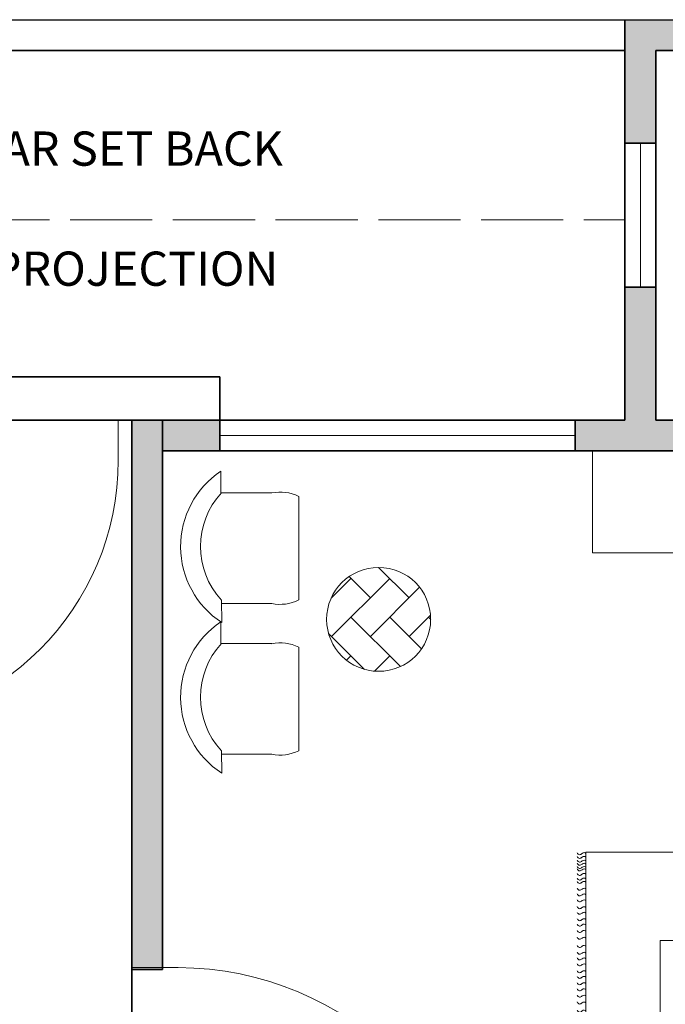
# Model space of a CAD drawing. Units: inches. Extents: x 0 to 4258, y 0 to 3769.
# Tile 27 of 30: x 3845 to 3940, y 3513 to 3657. Entities that reach past the tile are written whole.
import ezdxf

# ---------------------------------------------------------------- set-up
doc = ezdxf.new("R2010")
doc.units = ezdxf.units.IN
doc.header["$MEASUREMENT"] = 0
doc.linetypes.add('ACAD_ISO02W100', pattern=[15, 12, -3])
doc.layers.get('0').update_dxf_attribs({"color": 16})
for name, color, linetype, lineweight in [('A-ANNO-TEXT', 250, 'Continuous', 18), ('A-FLOR-OVHD', 150, 'ACAD_ISO02W100', 13), ('A-WALL-PATT', 16, 'Continuous', 13), ('C-PROP', 150, 'Continuous', 25), ('doors', 250, 'Continuous', 18), ('furniture', 13, 'Continuous', 18), ('walls', 251, 'Continuous', 35), ('windows', 121, 'Continuous', 18)]:
    doc.layers.add(name, color=color, linetype=linetype, lineweight=lineweight)
doc.styles.get("Standard").update_dxf_attribs({"font": 'arial.ttf'})

# ---------------------------------------------------------------- blocks, each defined once
blk = doc.blocks.new('CARPET')
at = {"layer": 'furniture'}
for p, q in [((-51.53, -98.11), (-51.53, -55.12)), ((-51.53, -55.12), (-41.27, -55.12)), ((36, -55.12), (51.55, -55.12)), ((51.55, -55.12), (51.55, -98.11)), ((51.55, -98.11), (-51.53, -98.11))]:
    blk.add_line(p, q, dxfattribs=at)
for points, knots in [([(-53.37, -55.99), (-53.22, -55.8), (-52.9, -55.41), (-52.34, -55.8), (-51.89, -56.08), (-51.65, -55.91), (-51.53, -55.83)], [0, 0, 0, 0, 0.653278, 1.290138, 1.740457, 2.114451, 2.114451, 2.114451, 2.114451]), ([(53.37, -55.99), (53.22, -55.8), (52.9, -55.41), (52.34, -55.8), (51.89, -56.08), (51.65, -55.91), (51.53, -55.83)], [0, 0, 0, 0, 0.653278, 1.290138, 1.740457, 2.114451, 2.114451, 2.114451, 2.114451]), ([(-53.37, -57.26), (-53.22, -57.07), (-52.9, -56.67), (-52.34, -57.07), (-51.89, -57.35), (-51.65, -57.17), (-51.53, -57.1)], [0, 0, 0, 0, 0.653278, 1.290138, 1.740457, 2.114451, 2.114451, 2.114451, 2.114451]), ([(53.37, -57.26), (53.22, -57.07), (52.9, -56.67), (52.34, -57.07), (51.89, -57.35), (51.65, -57.17), (51.53, -57.1)], [0, 0, 0, 0, 0.653278, 1.290138, 1.740457, 2.114451, 2.114451, 2.114451, 2.114451]), ([(-53.37, -58.59), (-53.22, -58.4), (-52.9, -58.01), (-52.34, -58.4), (-51.89, -58.68), (-51.65, -58.5), (-51.53, -58.43)], [0, 0, 0, 0, 0.653278, 1.290138, 1.740457, 2.114451, 2.114451, 2.114451, 2.114451]), ([(-53.37, -59.78), (-53.22, -59.58), (-52.9, -59.19), (-52.34, -59.58), (-51.89, -59.86), (-51.65, -59.69), (-51.53, -59.61)], [0, 0, 0, 0, 0.653278, 1.290138, 1.740457, 2.114451, 2.114451, 2.114451, 2.114451]), ([(53.37, -58.59), (53.22, -58.4), (52.9, -58.01), (52.34, -58.4), (51.89, -58.68), (51.65, -58.5), (51.53, -58.43)], [0, 0, 0, 0, 0.653278, 1.290138, 1.740457, 2.114451, 2.114451, 2.114451, 2.114451]), ([(53.37, -59.78), (53.22, -59.58), (52.9, -59.19), (52.34, -59.58), (51.89, -59.86), (51.65, -59.69), (51.53, -59.61)], [0, 0, 0, 0, 0.653278, 1.290138, 1.740457, 2.114451, 2.114451, 2.114451, 2.114451]), ([(-53.37, -61.22), (-53.22, -61.02), (-52.9, -60.63), (-52.34, -61.02), (-51.89, -61.3), (-51.65, -61.13), (-51.53, -61.05)], [0, 0, 0, 0, 0.653278, 1.290138, 1.740457, 2.114451, 2.114451, 2.114451, 2.114451]), ([(53.37, -61.22), (53.22, -61.02), (52.9, -60.63), (52.34, -61.02), (51.89, -61.3), (51.65, -61.13), (51.53, -61.05)], [0, 0, 0, 0, 0.653278, 1.290138, 1.740457, 2.114451, 2.114451, 2.114451, 2.114451]), ([(-53.37, -62.44), (-53.22, -62.25), (-52.9, -61.86), (-52.34, -62.25), (-51.89, -62.53), (-51.65, -62.36), (-51.53, -62.28)], [0, 0, 0, 0, 0.653278, 1.290138, 1.740457, 2.114451, 2.114451, 2.114451, 2.114451]), ([(-53.37, -63.63), (-53.22, -63.43), (-52.9, -63.04), (-52.34, -63.43), (-51.89, -63.72), (-51.65, -63.54), (-51.53, -63.46)], [0, 0, 0, 0, 0.653278, 1.290138, 1.740457, 2.114451, 2.114451, 2.114451, 2.114451]), ([(53.37, -62.44), (53.22, -62.25), (52.9, -61.86), (52.34, -62.25), (51.89, -62.53), (51.65, -62.36), (51.53, -62.28)], [0, 0, 0, 0, 0.653278, 1.290138, 1.740457, 2.114451, 2.114451, 2.114451, 2.114451]), ([(53.37, -63.63), (53.22, -63.43), (52.9, -63.04), (52.34, -63.43), (51.89, -63.72), (51.65, -63.54), (51.53, -63.46)], [0, 0, 0, 0, 0.653278, 1.290138, 1.740457, 2.114451, 2.114451, 2.114451, 2.114451]), ([(-53.37, -65.07), (-53.22, -64.87), (-52.9, -64.48), (-52.34, -64.87), (-51.89, -65.15), (-51.65, -64.98), (-51.53, -64.9)], [0, 0, 0, 0, 0.653278, 1.290138, 1.740457, 2.114451, 2.114451, 2.114451, 2.114451]), ([(53.37, -65.07), (53.22, -64.87), (52.9, -64.48), (52.34, -64.87), (51.89, -65.15), (51.65, -64.98), (51.53, -64.9)], [0, 0, 0, 0, 0.653278, 1.290138, 1.740457, 2.114451, 2.114451, 2.114451, 2.114451]), ([(-53.37, -66.76), (-53.22, -66.56), (-52.9, -66.17), (-52.34, -66.56), (-51.89, -66.84), (-51.65, -66.67), (-51.53, -66.59)], [0, 0, 0, 0, 0.653278, 1.290138, 1.740457, 2.114451, 2.114451, 2.114451, 2.114451]), ([(-53.37, -68.2), (-53.22, -68), (-52.9, -67.61), (-52.34, -68), (-51.89, -68.28), (-51.65, -68.11), (-51.53, -68.03)], [0, 0, 0, 0, 0.653278, 1.290138, 1.740457, 2.114451, 2.114451, 2.114451, 2.114451]), ([(53.37, -66.76), (53.22, -66.56), (52.9, -66.17), (52.34, -66.56), (51.89, -66.84), (51.65, -66.67), (51.53, -66.59)], [0, 0, 0, 0, 0.653278, 1.290138, 1.740457, 2.114451, 2.114451, 2.114451, 2.114451]), ([(53.37, -68.2), (53.22, -68), (52.9, -67.61), (52.34, -68), (51.89, -68.28), (51.65, -68.11), (51.53, -68.03)], [0, 0, 0, 0, 0.653278, 1.290138, 1.740457, 2.114451, 2.114451, 2.114451, 2.114451]), ([(-53.37, -69.53), (-53.22, -69.33), (-52.9, -68.94), (-52.34, -69.33), (-51.89, -69.61), (-51.65, -69.44), (-51.53, -69.36)], [0, 0, 0, 0, 0.653278, 1.290138, 1.740457, 2.114451, 2.114451, 2.114451, 2.114451]), ([(53.37, -69.53), (53.22, -69.33), (52.9, -68.94), (52.34, -69.33), (51.89, -69.61), (51.65, -69.44), (51.53, -69.36)], [0, 0, 0, 0, 0.653278, 1.290138, 1.740457, 2.114451, 2.114451, 2.114451, 2.114451]), ([(-53.37, -70.79), (-53.22, -70.6), (-52.9, -70.21), (-52.34, -70.6), (-51.89, -70.88), (-51.65, -70.7), (-51.53, -70.63)], [0, 0, 0, 0, 0.653278, 1.290138, 1.740457, 2.114451, 2.114451, 2.114451, 2.114451]), ([(-53.37, -72.12), (-53.22, -71.93), (-52.9, -71.54), (-52.34, -71.93), (-51.89, -72.21), (-51.65, -72.04), (-51.53, -71.96)], [0, 0, 0, 0, 0.653278, 1.290138, 1.740457, 2.114451, 2.114451, 2.114451, 2.114451]), ([(53.37, -70.79), (53.22, -70.6), (52.9, -70.21), (52.34, -70.6), (51.89, -70.88), (51.65, -70.7), (51.53, -70.63)], [0, 0, 0, 0, 0.653278, 1.290138, 1.740457, 2.114451, 2.114451, 2.114451, 2.114451]), ([(53.37, -72.12), (53.22, -71.93), (52.9, -71.54), (52.34, -71.93), (51.89, -72.21), (51.65, -72.04), (51.53, -71.96)], [0, 0, 0, 0, 0.653278, 1.290138, 1.740457, 2.114451, 2.114451, 2.114451, 2.114451]), ([(-53.37, -73.31), (-53.22, -73.11), (-52.9, -72.72), (-52.34, -73.11), (-51.89, -73.4), (-51.65, -73.22), (-51.53, -73.14)], [0, 0, 0, 0, 0.653278, 1.290138, 1.740457, 2.114451, 2.114451, 2.114451, 2.114451]), ([(53.37, -73.31), (53.22, -73.11), (52.9, -72.72), (52.34, -73.11), (51.89, -73.4), (51.65, -73.22), (51.53, -73.14)], [0, 0, 0, 0, 0.653278, 1.290138, 1.740457, 2.114451, 2.114451, 2.114451, 2.114451]), ([(-53.37, -74.75), (-53.22, -74.55), (-52.9, -74.16), (-52.34, -74.55), (-51.89, -74.83), (-51.65, -74.66), (-51.53, -74.58)], [0, 0, 0, 0, 0.653278, 1.290138, 1.740457, 2.114451, 2.114451, 2.114451, 2.114451]), ([(-53.37, -75.98), (-53.22, -75.78), (-52.9, -75.39), (-52.34, -75.78), (-51.89, -76.06), (-51.65, -75.89), (-51.53, -75.81)], [0, 0, 0, 0, 0.653278, 1.290138, 1.740457, 2.114451, 2.114451, 2.114451, 2.114451]), ([(53.37, -74.75), (53.22, -74.55), (52.9, -74.16), (52.34, -74.55), (51.89, -74.83), (51.65, -74.66), (51.53, -74.58)], [0, 0, 0, 0, 0.653278, 1.290138, 1.740457, 2.114451, 2.114451, 2.114451, 2.114451]), ([(53.37, -75.98), (53.22, -75.78), (52.9, -75.39), (52.34, -75.78), (51.89, -76.06), (51.65, -75.89), (51.53, -75.81)], [0, 0, 0, 0, 0.653278, 1.290138, 1.740457, 2.114451, 2.114451, 2.114451, 2.114451]), ([(-53.37, -77.16), (-53.22, -76.96), (-52.9, -76.57), (-52.34, -76.96), (-51.89, -77.25), (-51.65, -77.07), (-51.53, -76.99)], [0, 0, 0, 0, 0.653278, 1.290138, 1.740457, 2.114451, 2.114451, 2.114451, 2.114451]), ([(-53.37, -78.6), (-53.22, -78.4), (-52.9, -78.01), (-52.34, -78.4), (-51.89, -78.68), (-51.65, -78.51), (-51.53, -78.43)], [0, 0, 0, 0, 0.653278, 1.290138, 1.740457, 2.114451, 2.114451, 2.114451, 2.114451]), ([(53.37, -77.16), (53.22, -76.96), (52.9, -76.57), (52.34, -76.96), (51.89, -77.25), (51.65, -77.07), (51.53, -76.99)], [0, 0, 0, 0, 0.653278, 1.290138, 1.740457, 2.114451, 2.114451, 2.114451, 2.114451]), ([(53.37, -78.6), (53.22, -78.4), (52.9, -78.01), (52.34, -78.4), (51.89, -78.68), (51.65, -78.51), (51.53, -78.43)], [0, 0, 0, 0, 0.653278, 1.290138, 1.740457, 2.114451, 2.114451, 2.114451, 2.114451]), ([(-53.37, -80.29), (-53.22, -80.09), (-52.9, -79.7), (-52.34, -80.09), (-51.89, -80.37), (-51.65, -80.2), (-51.53, -80.12)], [0, 0, 0, 0, 0.653278, 1.290138, 1.740457, 2.114451, 2.114451, 2.114451, 2.114451]), ([(53.37, -80.29), (53.22, -80.09), (52.9, -79.7), (52.34, -80.09), (51.89, -80.37), (51.65, -80.2), (51.53, -80.12)], [0, 0, 0, 0, 0.653278, 1.290138, 1.740457, 2.114451, 2.114451, 2.114451, 2.114451]), ([(-53.37, -81.73), (-53.22, -81.53), (-52.9, -81.14), (-52.34, -81.53), (-51.89, -81.81), (-51.65, -81.64), (-51.53, -81.56)], [0, 0, 0, 0, 0.653278, 1.290138, 1.740457, 2.114451, 2.114451, 2.114451, 2.114451]), ([(53.37, -81.73), (53.22, -81.53), (52.9, -81.14), (52.34, -81.53), (51.89, -81.81), (51.65, -81.64), (51.53, -81.56)], [0, 0, 0, 0, 0.653278, 1.290138, 1.740457, 2.114451, 2.114451, 2.114451, 2.114451]), ([(-53.37, -83.06), (-53.22, -82.86), (-52.9, -82.47), (-52.34, -82.86), (-51.89, -83.14), (-51.65, -82.97), (-51.53, -82.89)], [0, 0, 0, 0, 0.653278, 1.290138, 1.740457, 2.114451, 2.114451, 2.114451, 2.114451]), ([(-53.37, -84.18), (-53.22, -83.99), (-52.9, -83.6), (-52.34, -83.99), (-51.89, -84.27), (-51.65, -84.09), (-51.53, -84.02)], [0, 0, 0, 0, 0.653278, 1.290138, 1.740457, 2.114451, 2.114451, 2.114451, 2.114451]), ([(53.37, -83.06), (53.22, -82.86), (52.9, -82.47), (52.34, -82.86), (51.89, -83.14), (51.65, -82.97), (51.53, -82.89)], [0, 0, 0, 0, 0.653278, 1.290138, 1.740457, 2.114451, 2.114451, 2.114451, 2.114451]), ([(53.37, -84.18), (53.22, -83.99), (52.9, -83.6), (52.34, -83.99), (51.89, -84.27), (51.65, -84.09), (51.53, -84.02)], [0, 0, 0, 0, 0.653278, 1.290138, 1.740457, 2.114451, 2.114451, 2.114451, 2.114451]), ([(-53.37, -85.51), (-53.22, -85.32), (-52.9, -84.93), (-52.34, -85.32), (-51.89, -85.6), (-51.65, -85.42), (-51.53, -85.35)], [0, 0, 0, 0, 0.653278, 1.290138, 1.740457, 2.114451, 2.114451, 2.114451, 2.114451]), ([(-53.37, -86.7), (-53.22, -86.5), (-52.9, -86.11), (-52.34, -86.5), (-51.89, -86.78), (-51.65, -86.61), (-51.53, -86.53)], [0, 0, 0, 0, 0.653278, 1.290138, 1.740457, 2.114451, 2.114451, 2.114451, 2.114451]), ([(53.37, -85.51), (53.22, -85.32), (52.9, -84.93), (52.34, -85.32), (51.89, -85.6), (51.65, -85.42), (51.53, -85.35)], [0, 0, 0, 0, 0.653278, 1.290138, 1.740457, 2.114451, 2.114451, 2.114451, 2.114451]), ([(53.37, -86.7), (53.22, -86.5), (52.9, -86.11), (52.34, -86.5), (51.89, -86.78), (51.65, -86.61), (51.53, -86.53)], [0, 0, 0, 0, 0.653278, 1.290138, 1.740457, 2.114451, 2.114451, 2.114451, 2.114451]), ([(-53.37, -88.14), (-53.22, -87.94), (-52.9, -87.55), (-52.34, -87.94), (-51.89, -88.22), (-51.65, -88.05), (-51.53, -87.97)], [0, 0, 0, 0, 0.653278, 1.290138, 1.740457, 2.114451, 2.114451, 2.114451, 2.114451]), ([(53.37, -88.14), (53.22, -87.94), (52.9, -87.55), (52.34, -87.94), (51.89, -88.22), (51.65, -88.05), (51.53, -87.97)], [0, 0, 0, 0, 0.653278, 1.290138, 1.740457, 2.114451, 2.114451, 2.114451, 2.114451]), ([(-53.37, -89.36), (-53.22, -89.17), (-52.9, -88.78), (-52.34, -89.17), (-51.89, -89.45), (-51.65, -89.28), (-51.53, -89.2)], [0, 0, 0, 0, 0.653278, 1.290138, 1.740457, 2.114451, 2.114451, 2.114451, 2.114451]), ([(-53.37, -90.55), (-53.22, -90.35), (-52.9, -89.96), (-52.34, -90.35), (-51.89, -90.64), (-51.65, -90.46), (-51.53, -90.38)], [0, 0, 0, 0, 0.653278, 1.290138, 1.740457, 2.114451, 2.114451, 2.114451, 2.114451]), ([(53.37, -89.36), (53.22, -89.17), (52.9, -88.78), (52.34, -89.17), (51.89, -89.45), (51.65, -89.28), (51.53, -89.2)], [0, 0, 0, 0, 0.653278, 1.290138, 1.740457, 2.114451, 2.114451, 2.114451, 2.114451]), ([(53.37, -90.55), (53.22, -90.35), (52.9, -89.96), (52.34, -90.35), (51.9, -90.63), (51.66, -90.47), (51.55, -90.4)], [0, 0, 0, 0, 0.653278, 1.290138, 1.740457, 2.0926, 2.0926, 2.0926, 2.0926]), ([(-53.37, -91.99), (-53.22, -91.79), (-52.9, -91.4), (-52.34, -91.79), (-51.89, -92.07), (-51.65, -91.9), (-51.53, -91.82)], [0, 0, 0, 0, 0.653278, 1.290138, 1.740457, 2.114451, 2.114451, 2.114451, 2.114451]), ([(-53.37, -92.69), (-53.22, -92.48), (-52.9, -92.08), (-52.35, -92.49), (-51.89, -92.77), (-51.65, -92.6), (-51.53, -92.52)], [0, 0, 0, 0, 0.663904, 1.307406, 1.757725, 2.131719, 2.131719, 2.131719, 2.131719]), ([(53.37, -91.99), (53.22, -91.79), (52.9, -91.4), (52.34, -91.79), (51.9, -92.07), (51.66, -91.91), (51.55, -91.83)], [0, 0, 0, 0, 0.653278, 1.290138, 1.740457, 2.0926, 2.0926, 2.0926, 2.0926]), ([(53.37, -92.69), (53.22, -92.49), (52.9, -92.09), (52.34, -92.49), (51.9, -92.77), (51.66, -92.61), (51.55, -92.53)], [0, 0, 0, 0, 0.656792, 1.295826, 1.746145, 2.098292, 2.098292, 2.098292, 2.098292]), ([(-53.37, -93.61), (-53.22, -93.42), (-52.9, -93.03), (-52.34, -93.42), (-51.89, -93.7), (-51.65, -93.52), (-51.53, -93.45)], [0, 0, 0, 0, 0.653278, 1.290138, 1.740457, 2.114451, 2.114451, 2.114451, 2.114451]), ([(-53.37, -94.55), (-53.22, -94.35), (-52.9, -93.96), (-52.34, -94.35), (-51.89, -94.63), (-51.65, -94.46), (-51.53, -94.38)], [0, 0, 0, 0, 0.653278, 1.290138, 1.740457, 2.114451, 2.114451, 2.114451, 2.114451]), ([(-53.37, -95.05), (-53.22, -94.85), (-52.9, -94.46), (-52.34, -94.85), (-51.89, -95.14), (-51.65, -94.96), (-51.53, -94.88)], [0, 0, 0, 0, 0.653278, 1.290138, 1.740457, 2.114451, 2.114451, 2.114451, 2.114451]), ([(53.37, -93.66), (53.22, -93.46), (52.9, -93.07), (52.34, -93.46), (51.9, -93.74), (51.66, -93.58), (51.55, -93.5)], [0, 0, 0, 0, 0.653278, 1.290138, 1.740457, 2.0926, 2.0926, 2.0926, 2.0926]), ([(53.37, -94.59), (53.22, -94.4), (52.9, -94.01), (52.34, -94.4), (51.9, -94.68), (51.66, -94.51), (51.55, -94.44)], [0, 0, 0, 0, 0.653278, 1.290138, 1.740457, 2.0926, 2.0926, 2.0926, 2.0926]), ([(53.37, -95.1), (53.22, -94.9), (52.9, -94.51), (52.34, -94.9), (51.9, -95.18), (51.66, -95.02), (51.55, -94.94)], [0, 0, 0, 0, 0.653278, 1.290138, 1.740457, 2.0926, 2.0926, 2.0926, 2.0926]), ([(-53.37, -95.73), (-53.22, -95.54), (-52.9, -95.15), (-52.34, -95.54), (-51.89, -95.82), (-51.65, -95.65), (-51.53, -95.57)], [0, 0, 0, 0, 0.653278, 1.290138, 1.740457, 2.114451, 2.114451, 2.114451, 2.114451]), ([(-53.37, -96.38), (-53.22, -96.18), (-52.9, -95.79), (-52.34, -96.18), (-51.89, -96.47), (-51.65, -96.29), (-51.53, -96.21)], [0, 0, 0, 0, 0.653278, 1.290138, 1.740457, 2.114451, 2.114451, 2.114451, 2.114451]), ([(-53.37, -97.17), (-53.22, -96.98), (-52.9, -96.59), (-52.34, -96.98), (-51.89, -97.26), (-51.65, -97.08), (-51.53, -97.01)], [0, 0, 0, 0, 0.653278, 1.290138, 1.740457, 2.114451, 2.114451, 2.114451, 2.114451]), ([(53.37, -95.78), (53.22, -95.58), (52.9, -95.19), (52.34, -95.58), (51.89, -95.86), (51.65, -95.69), (51.53, -95.61)], [0, 0, 0, 0, 0.653278, 1.290138, 1.740457, 2.114451, 2.114451, 2.114451, 2.114451]), ([(53.37, -96.43), (53.22, -96.23), (52.9, -95.84), (52.34, -96.23), (51.89, -96.51), (51.65, -96.34), (51.53, -96.26)], [0, 0, 0, 0, 0.653278, 1.290138, 1.740457, 2.114451, 2.114451, 2.114451, 2.114451]), ([(53.37, -97.22), (53.22, -97.02), (52.9, -96.63), (52.34, -97.02), (51.89, -97.3), (51.65, -97.13), (51.53, -97.05)], [0, 0, 0, 0, 0.653278, 1.290138, 1.740457, 2.114451, 2.114451, 2.114451, 2.114451]), ([(-53.37, -97.99), (-53.22, -97.79), (-52.9, -97.4), (-52.34, -97.79), (-51.89, -98.08), (-51.65, -97.9), (-51.53, -97.82)], [0, 0, 0, 0, 0.653278, 1.290138, 1.740457, 2.114451, 2.114451, 2.114451, 2.114451]), ([(53.37, -97.99), (53.22, -97.79), (52.9, -97.4), (52.34, -97.79), (51.89, -98.08), (51.65, -97.9), (51.53, -97.82)], [0, 0, 0, 0, 0.653278, 1.290138, 1.740457, 2.114451, 2.114451, 2.114451, 2.114451])]:
    blk.add_open_spline(points, degree=3, knots=knots, dxfattribs=at)
blk = doc.blocks.new('A$C58D270C6')
at = {"layer": 'furniture'}
for p, q in [((9.09, 124.13), (9.09, 108.87)), ((1.46, 116.5), (16.73, 116.5)), ((14.97, 94.84), (24.62, 107.92)), ((24.62, 94.93), (24.62, 107.92)), ((42.08, 108), (42.08, 36)), ((14.97, 94.93), (24.62, 94.93)), ((14.97, 94.84), (14.97, 36)), ((16.22, 94.93), (16.22, 36)), ((9.25, 36), (9.25, 20.74)), ((1.62, 28.37), (16.88, 28.37))]:
    blk.add_line(p, q, dxfattribs=at)
for points in [[(18.5, 108), (18.34, 124.13), (-0.16, 124.13), (0, 108)], [(0, 108), (77.91, 108), (77.91, 36), (0, 36)], [(4.09, 94.93), (14.97, 94.93), (14.97, 73.83), (4.09, 73.83)], [(4.09, 65.23), (14.97, 65.23), (14.97, 44.13), (4.09, 44.13)], [(18.65, 19.87), (18.5, 36), (0, 36), (0.16, 19.87)]]:
    blk.add_lwpolyline(points, close=True, dxfattribs=at)
for centre in [(9.09, 116.5), (9.25, 28.37)]:
    blk.add_circle(centre, 5.95, dxfattribs=at)
at = {"layer": 'furniture', "xscale": 0.9312884925094044, "yscale": 0.9312884925094044, "zscale": 0.9312884925094044, "rotation": 90}
blk.add_blockref('CARPET', (3.79, 74.47), dxfattribs=at)
blk = doc.blocks.new('*U23')
for p, q in [((0, 0), (0, -6)), ((40, 0), (40, -6))]:
    blk.add_line(p, q)
blk.add_lwpolyline([(0, 0), (0, 40), (1.75, 40), (1.75, 0)], close=True)
blk.add_arc((0, 0), 40, 0, 90)
blk = doc.blocks.new('SEATING-TWO-CHAIRS-AND-TABLE')
h = blk.add_hatch()
h.set_pattern_fill('AR-HBONE', color=256, angle=90)
h.set_pattern_definition([(135, (3403.542, -4056.0025), (-5.6568542, 3e-16), [12, -4]), (225, (3400.7137, -4053.174), (-5.6568542, 8e-16), [12, -4])])
h.paths.add_polyline_path([(7.59, 14.04, 1), (7.59, 29.23, 1)])
for p, q in [((30.53, 40.83), (30.5, 44.11)), ((19.25, 25.7), (19.25, 40.83)), ((23.18, 41.34), (30.53, 41.34)), ((23.18, 25.19), (30.53, 25.19)), ((30.63, 22.02), (30.63, 25.19)), ((30.53, 18.81), (30.5, 22.09)), ((19.25, 3.68), (19.25, 18.81)), ((23.18, 19.32), (30.53, 19.32)), ((23.18, 3.17), (30.53, 3.17)), ((30.63, 0), (30.63, 3.17))]:
    blk.add_line(p, q)
blk.add_circle((7.59, 21.64), 7.59)
for centre, radius, start, end in [((23.25, 33.02), 13.25, 303.8239, 56.829), ((21.94, 35.53), 5.94, 77.9198, 116.8624), ((22.13, 33.01), 11.48, 317.0375, 42.9625), ((21.94, 31), 5.94, 243.1376, 282.0802), ((23.25, 11.01), 13.25, 303.8239, 56.829), ((21.94, 13.51), 5.94, 77.9198, 116.8624), ((22.13, 10.99), 11.48, 317.0375, 42.9625), ((21.94, 8.98), 5.94, 243.1376, 282.0802)]:
    blk.add_arc(centre, radius, start, end)
blk = doc.blocks.new('WINDOW-21IN')
for p, q in [((0, 21.04), (0, 0)), ((2.25, 21.04), (2.25, 0)), ((4.5, 21.04), (4.5, 0))]:
    blk.add_line(p, q)
blk = doc.blocks.new('TV-CONSOLE-CABINET')
for p, q in [((0, 0), (0, 64.44)), ((0, 64.44), (14.9, 64.44)), ((14.9, 0), (0, 0))]:
    blk.add_line(p, q)

msp = doc.modelspace()

# ---------------------------------------------------------------- hatches: boundary and pattern name
at = {"layer": 'A-WALL-PATT'}
h = msp.add_hatch(color=256, dxfattribs=at)
h.dxf.hatch_style = 1
h.paths.add_polyline_path([(3866.304, 3343.984), (3861.804, 3343.984), (3861.804, 3251.848), (3866.304, 3251.848)])
h.paths.add_polyline_path([(3881.946, 3330.642), (3866.304, 3330.642), (3866.304, 3326.142), (3881.946, 3326.142)])
h.paths.add_polyline_path([(4038.804, 3656.793), (3933.804, 3656.793), (3933.804, 3638.769), (3938.304, 3638.769), (3938.304, 3652.293), (4034.304, 3652.293), (4034.304, 3260.793), (4030.207, 3260.793), (4030.207, 3256.293), (4038.804, 3256.293)])
h = msp.add_hatch(color=256, dxfattribs=at)
h.dxf.hatch_style = 1
h.paths.add_polyline_path([(4005.754, 3597.57, -0.0071857), (4005.764, 3598.293), (3938.304, 3598.293), (3938.304, 3617.728), (3933.804, 3617.728), (3933.804, 3598.293), (3926.508, 3598.293), (3926.508, 3593.793), (4005.754, 3593.793)])
h = msp.add_hatch(color=256, dxfattribs=at)
h.dxf.hatch_style = 1
h.paths.add_polyline_path([(3866.304, 3598.293), (3861.804, 3598.293), (3861.804, 3518.033), (3866.304, 3518.033), (3866.304, 3518.314)])
h = msp.add_hatch(color=256, dxfattribs=at)
h.dxf.hatch_style = 1
h.paths.add_polyline_path([(3874.654, 3598.293), (3866.304, 3598.293), (3866.304, 3593.793), (3874.654, 3593.793)])

# ---------------------------------------------------------------- linework, layer by layer
at = {"layer": 'A-FLOR-OVHD'}
msp.add_line((3777.804, 3627.543), (3933.804, 3627.543), dxfattribs=at)
at = {"layer": 'C-PROP'}
for p, q in [((3678.804, 3656.793), (4038.804, 3656.793)), ((3777.804, 3656.793), (3933.804, 3656.793)), ((3777.804, 3652.293), (3933.804, 3652.293))]:
    msp.add_line(p, q, dxfattribs=at)
at = {"layer": 'walls'}
for p, q in [((3933.804, 3656.793), (3933.804, 3598.293)), ((3777.804, 3652.293), (3933.804, 3652.293)), ((3938.304, 3652.293), (3938.304, 3598.293)), ((3938.304, 3652.293), (4034.304, 3652.293)), ((3933.804, 3638.769), (3938.304, 3638.769)), ((3933.804, 3617.728), (3938.304, 3617.728)), ((3801.818, 3604.636), (3874.654, 3604.636)), ((3874.654, 3604.636), (3874.654, 3598.293)), ((3819.804, 3598.293), (3861.804, 3598.293)), ((3861.804, 3598.293), (3861.804, 3163.293)), ((3861.804, 3598.293), (3933.804, 3598.293)), ((3866.304, 3598.293), (3866.304, 3518.314)), ((3874.654, 3598.293), (3874.654, 3593.793)), ((3926.508, 3598.293), (3926.508, 3593.793)), ((3938.304, 3598.293), (4005.764, 3598.293)), ((3866.304, 3593.793), (4034.304, 3593.793)), ((3866.304, 3518.033), (3866.304, 3518.314)), ((3861.804, 3518.033), (3866.304, 3518.033))]:
    msp.add_line(p, q, dxfattribs=at)
at = {"layer": 'windows'}
for p, q in [((3874.654, 3598.293), (3926.508, 3598.293)), ((3874.654, 3596.043), (3926.508, 3596.043)), ((3874.654, 3593.793), (3926.508, 3593.793))]:
    msp.add_line(p, q, dxfattribs=at)

# ---------------------------------------------------------------- block references
at = {"layer": 'doors'}
for p, xscale, yscale, zscale, rotation in [((3820.752, 3592.431), -0.9769813032789267, 0.9769813032789267, 0.9769813032789267, 180), ((3868.56, 3473.274), -1.125993190768673, 1.125993190768673, 1.125993190768673, 270)]:
    msp.add_blockref('*U23', p, dxfattribs=dict(at, xscale=xscale, yscale=yscale, zscale=zscale, rotation=rotation))
at = {"layer": 'furniture'}
for name, p, rotation in [('TV-CONSOLE-CABINET', (3993.494, 3578.897), 89.9999999999983), ('SEATING-TWO-CHAIRS-AND-TABLE', (3905.434, 3590.831), 180)]:
    msp.add_blockref(name, p, dxfattribs=dict(at, rotation=rotation))
at = {"layer": 'furniture', "xscale": 0.7500000390647866, "yscale": 0.7500000390647866, "zscale": 0.7500000390647866, "rotation": 90}
msp.add_blockref('A$C58D270C6', (4019.941, 3463.822), dxfattribs=at)
at = {"layer": 'windows'}
msp.add_blockref('WINDOW-21IN', (3933.804, 3617.728), dxfattribs=at)

# ---------------------------------------------------------------- texts
at = {"layer": 'A-ANNO-TEXT'}
for s, p in [("5' WIDE REAR SET BACK", (3808.998, 3635.463)), ('3\'-6" WIDE PROJECTION', (3806.567, 3617.92))]:
    msp.add_text(s, height=5, dxfattribs=at).set_placement(p)

doc.saveas('drawing.dxf')
